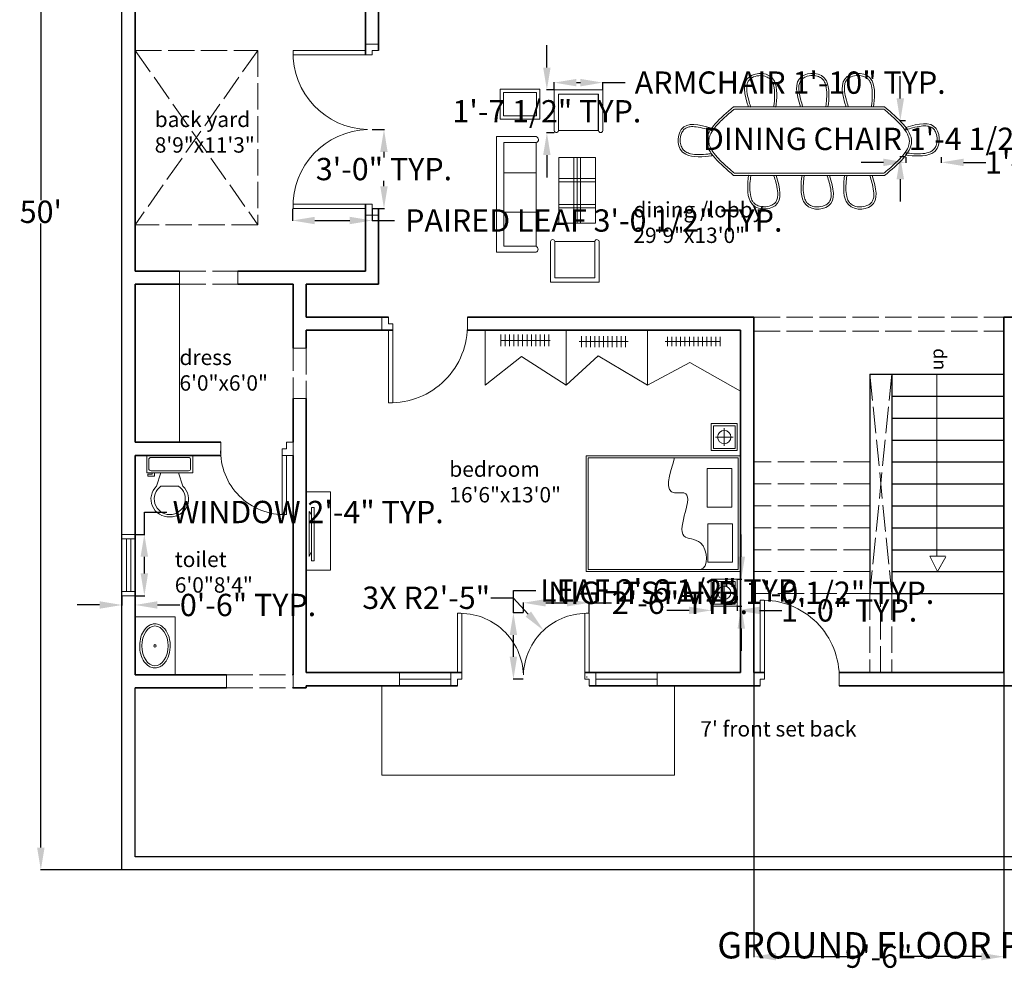
# Model space of a CAD drawing. Units: inches. Extents: x 29 to 4581, y 6 to 2196.
# Tile 1 of 3: x 3825 to 4274, y 1514 to 1948. Entities that reach past the tile are written whole.
import ezdxf

# ---------------------------------------------------------------- set-up
doc = ezdxf.new("R2010")
doc.units = ezdxf.units.IN
doc.header["$MEASUREMENT"] = 0
doc.linetypes.add('ACAD_ISO02W100', pattern=[15, 12, -3])
for name, color, linetype, lineweight in [('A-ANNO-DIMS', 2, 'Continuous', 18), ('A-ANNO-SYMB', 7, 'Continuous', 18), ('A-ANNO-TEXT', 7, 'Continuous', 25), ('A-DOOR', 3, 'Continuous', 18), ('A-EQPM', 9, 'Continuous', 18), ('A-FLOR-CASE', 8, 'Continuous', 18), ('A-FLOR-CASE-PATT', 8, 'Continuous', 13), ('A-FLOR-FIXT', 9, 'Continuous', 18), ('A-FLOR-OPEN', 8, 'ACAD_ISO02W100', 13), ('A-FLOR-STRS', 7, 'Continuous', 25), ('A-FLOR-STRS-HIDN', 8, 'ACAD_ISO02W100', 18), ('A-GLAZ', 4, 'Continuous', 18), ('A-WALL', 7, 'Continuous', 35), ('A-WALL-OVHD', 8, 'ACAD_ISO02W100', 18), ('C-PROP', 8, 'Continuous', 25), ('L-HRDS', 8, 'Continuous', 18)]:
    doc.layers.add(name, color=color, linetype=linetype, lineweight=lineweight)
doc.layers.add('A-AREA-IDEN', color=41, linetype='Continuous', lineweight=18, true_color=0xf4ee51)
doc.layers.add('A-FURN', color=31, linetype='Continuous', lineweight=18, true_color=0xfecc66)
doc.styles.get("Standard").update_dxf_attribs({"font": 'arial.ttf'})
doc.dimstyles.get("Standard").update_dxf_attribs({"dimtxt": 10.18, "dimasz": 10.18, "dimexe": 0.18, "dimexo": 0.0625, "dimgap": 0.09, "dimtad": 0, "dimtih": 1, "dimtoh": 1, "dimdec": 0, "dimzin": 0, "dimdsep": 46, "dimlunit": 3, "dimtxsty": 'Standard', "dimcen": 0.09, "dimadec": 0, "dimazin": 0, "dimtfac": 1, "dimtdec": 0, "dimtofl": 0, "dimtmove": 0, "dimatfit": 3, "dimfxl": 1, "dimtolj": 1, "dimtzin": 0, "dimarcsym": 0})

# ---------------------------------------------------------------- blocks, each defined once
blk = doc.blocks.new('*U2')
for p, q in [((9.5, -6), (9.5, -2)), ((-10, -8.5), (-8, -8.5)), ((-10, -9.5), (-10, -8.5)), ((-8, -8.5), (-8, -8)), ((-7, -8), (-7, -9.5)), ((-4, -8), (-6, -14)), ((4, -8), (6, -14)), ((-7, -9.5), (-10, -9.5)), ((4, -14), (-4, -14))]:
    blk.add_line(p, q)
blk.add_lwpolyline([(10.5, -8), (10.5, 0), (-10.5, 0), (-10.5, -8)], close=True)
for points in [[(-9.5, -2), (-9.5, -6)], [(8.5, -1), (-8.5, -1)], [(-8.5, -7), (8.5, -7)]]:
    blk.add_lwpolyline(points)
for centre, radius, start, end in [((-8.625, -1.875), 0.8839, 81.8699, 188.1301), ((8.625, -1.875), 0.8839, 351.8699, 98.1301), ((-8.625, -6.125), 0.8839, 171.869898, 278.1301), ((8.625, -6.125), 0.8839, 261.8699, 8.1301), ((-0.4772, -19.9188), 8.0953, 133.01722, 273.38), ((0.0374, -19.8731), 7.127, 124.50543, 269.7), ((-0.0373, -19.8731), 7.127, 270.3, 55.4946), ((0.4773, -19.9188), 8.0953, 266.62, 46.9828)]:
    blk.add_arc(centre, radius, start, end)
blk = doc.blocks.new('*D8')
at = {"layer": 'A-ANNO-DIMS', "color": 0, "lineweight": -2, "transparency": 16777216}
for p, q in [((3871.91, 2160.26), (3834.8, 2160.26)), ((3834.98, 2150.08), (3834.98, 1865.52)), ((3834.98, 1570.38), (3834.98, 1854.94)), ((3871.91, 1560.2), (3834.8, 1560.2))]:
    blk.add_line(p, q, dxfattribs=at)
at = {"layer": 'A-ANNO-DIMS', "color": 0, "transparency": 16777216}
for points in [[(3833.29, 2150.08), (3836.68, 2150.08), (3834.98, 2160.26)], [(3833.29, 1570.38), (3836.68, 1570.38), (3834.98, 1560.2)]]:
    blk.add_solid(points, dxfattribs=at)
at = {"layer": 'Defpoints', "color": 0, "transparency": 16777216}
for p in [(3834.98, 2160.26), (3871.98, 2160.26), (3871.98, 1560.2)]:
    blk.add_point(p, dxfattribs=at)
at = {"layer": 'A-ANNO-DIMS', "color": 0, "transparency": 16777216, "insert": (3834.98, 1860.23), "char_height": 10.18, "attachment_point": 5}
blk.add_mtext("\\A1;50'", dxfattribs=at)
blk = doc.blocks.new('CHAIR-DINING')
for p, q in [((2.81, 0.04), (1.75, 0.07)), ((13.32, 0.14), (14.31, 0))]:
    blk.add_line(p, q)
for points, knots in [([(1.75, 0.07), (0.01, 5.77), (-2.4, 15.72), (15.73, 16.36), (14.8, 3.53), (14.31, 0)], [1.303878, 1.303878, 1.303878, 1.303878, 15.362329, 26.918428, 34.974359, 34.974359, 34.974359, 34.974359]), ([(2.81, 0.04), (2.79, 0.11), (2.77, 0.18), (2.45, 1.22), (2.16, 2.19), (1.54, 4.52), (1.24, 5.86), (0.98, 8.1), (0.96, 9.04), (1.16, 10.48), (1.32, 11.03), (1.79, 11.99), (2.1, 12.41), (2.73, 12.97), (2.97, 13.14), (3.52, 13.47), (3.82, 13.62), (5.09, 14.12), (6.23, 14.34), (8.24, 14.32), (9.13, 14.17), (10.58, 13.61), (11.17, 13.26), (12, 12.49), (12.29, 12.14), (12.72, 11.45), (12.87, 11.13), (13.14, 10.42), (13.26, 10.03), (13.62, 8.47), (13.73, 7.13), (13.75, 4.38), (13.65, 2.98), (13.45, 1.15), (13.39, 0.63), (13.32, 0.14)], [1.038869, 1.038869, 1.038869, 1.038869, 1.209497, 1.209497, 3.62849, 3.62849, 7.242439, 7.242439, 10.256711, 10.256711, 12.544546, 12.544546, 14.832381, 14.832381, 15.973009, 15.973009, 17.113637, 17.113637, 20.41694, 20.41694, 23.018333, 23.018333, 25.159823, 25.159823, 26.539555, 26.539555, 27.513845, 27.513845, 28.488134, 28.488134, 31.162496, 31.162496, 33.836859, 33.836859, 34.97445, 34.97445, 34.97445, 34.97445])]:
    blk.add_open_spline(points, degree=3, knots=knots)
blk = doc.blocks.new('CHAIR-LOUNGE')
for points in [[(0, 0.82), (0, 19.42), (1.99, 19.42)], [(20.17, 19.42), (1.99, 19.42)], [(20.17, 19.42), (22.16, 19.42), (22.16, 0.82)], [(1.99, 17.47), (1.99, 0.82), (1.98, 0.82)], [(1.99, 17.47), (20.17, 17.47)], [(20.17, 0.82), (20.17, 17.47)]]:
    blk.add_lwpolyline(points)
blk.add_lwpolyline([(1.99, 17.47), (20.14, 17.47), (20.14, 0.87), (1.99, 0.87)], close=True)
for centre, radius, start, end in [((0.99, 1.01), 1.01, 190.5577, 7.8142), ((21.17, 1.03), 1.02, 191.625, 348.375)]:
    blk.add_arc(centre, radius, start, end)
blk = doc.blocks.new('DOOR-36IN')
for p, q in [((34.01, 0), (34.01, 36)), ((36.01, 3), (36.01, 36)), ((34.01, 0), (36.01, 0))]:
    blk.add_line(p, q)
blk.add_arc((35.01, 1), 35.01, 88.3634, 181.6366)
blk = doc.blocks.new('DOOR-36IN-PAIRED-LEAF')
for p, q in [((36.01, 2), (0.01, 2)), ((36.01, 2), (36.01, 0)), ((33.01, 0), (0.01, 0))]:
    blk.add_line(p, q)
blk.add_arc((35.01, 1), 35.01, 91.6366, 181.6366)
blk = doc.blocks.new('DOOR-30IN')
for p, q in [((0, 2), (30, 2)), ((0, 2), (0, 0)), ((3, 0), (30, 0))]:
    blk.add_line(p, q)
blk.add_arc((1, 1), 29.02, 358.0251, 91.9749)
blk = doc.blocks.new('DOOR-30IN-PAIRED-LEAF')
for p, q in [((28, 0), (28, 30)), ((30, 3), (30, 30)), ((28, 0), (30, 0))]:
    blk.add_line(p, q)
blk.add_arc((29, 1), 29.02, 88.0251, 178.0251)
blk = doc.blocks.new('WIN-24')
for p, q in [((6, 28), (0, 28)), ((6, 26), (0, 26)), ((2, 26), (2, 2)), ((4, 26), (4, 2)), ((6, 2), (0, 2)), ((6, 0), (0, 0))]:
    blk.add_line(p, q)
blk = doc.blocks.new('BASIN-OVAL')
blk.add_circle((10.07, 6.96), 0.572)
blk.add_ellipse((10.07, 6.96), major_axis=(9.07, 0), ratio=0.657752)
blk.add_open_spline([(20.13, 6.96), (20.13, 7.48), (20.05, 7.99), (19.74, 8.98), (19.5, 9.46), (18.6, 10.81), (17.74, 11.59), (15.67, 12.84), (14.47, 13.31), (11.89, 13.88), (10.52, 13.98), (7.83, 13.82), (6.51, 13.55), (4.11, 12.67), (3.03, 12.06), (1.49, 10.71), (0.93, 10.02), (0.24, 8.64), (0.05, 7.96), (-0.03, 6.59), (0.07, 5.9), (0.54, 4.6), (0.91, 3.98), (1.85, 2.86), (2.43, 2.36), (4.23, 1.16), (5.63, 0.61), (8.62, -0.01), (10.22, -0.08), (13.3, 0.28), (14.78, 0.7), (17.33, 1.99), (18.39, 2.86), (19.54, 4.5), (19.85, 5.16), (20.09, 6.22), (20.13, 6.59), (20.13, 6.96)], degree=3, knots=[0, 0, 0, 0, 0.206246, 0.206246, 0.412492, 0.412492, 0.829146, 0.829146, 1.245799, 1.245799, 1.662453, 1.662453, 2.079106, 2.079106, 2.495759, 2.495759, 2.824502, 2.824502, 3.099346, 3.099346, 3.37419, 3.37419, 3.649034, 3.649034, 3.923877, 3.923877, 4.405635, 4.405635, 4.887392, 4.887392, 5.369149, 5.369149, 5.850906, 5.850906, 6.134068, 6.134068, 6.283185, 6.283185, 6.283185, 6.283185])
blk = doc.blocks.new('NIGHTSTAND-NARROW')
for p, q in [((5.9, 10.31), (5.9, 2.16)), ((1.96, 6.19), (10.01, 6.19))]:
    blk.add_line(p, q)
for points in [[(0, 12.38), (11.8, 12.38), (11.8, 0), (0, 0)], [(1, 11.38), (10.8, 11.38), (10.8, 1), (1, 1)]]:
    blk.add_lwpolyline(points, close=True)
blk.add_circle((5.9, 6.19), 3.03)
blk = doc.blocks.new('*D22')
at = {"layer": 'A-ANNO-DIMS', "color": 0, "lineweight": -2, "transparency": 16777216}
for p, q in [((4226.82, 1911.89), (4226.82, 1922.07)), ((4229.23, 1901.71), (4226.64, 1901.71)), ((4229.23, 1885.22), (4226.64, 1885.22)), ((4226.82, 1875.04), (4226.82, 1864.86))]:
    blk.add_line(p, q, dxfattribs=at)
at = {"layer": 'A-ANNO-DIMS', "color": 0, "transparency": 16777216}
for points in [[(4225.13, 1911.89), (4228.52, 1911.89), (4226.82, 1901.71)], [(4225.13, 1875.04), (4228.52, 1875.04), (4226.82, 1885.22)]]:
    blk.add_solid(points, dxfattribs=at)
at = {"layer": 'Defpoints', "color": 0, "transparency": 16777216}
for p in [(4229.3, 1901.71), (4226.82, 1885.22), (4229.3, 1885.22)]:
    blk.add_point(p, dxfattribs=at)
at = {"layer": 'A-ANNO-DIMS', "color": 0, "transparency": 16777216, "insert": (4226.82, 1893.47), "char_height": 10.18, "attachment_point": 5}
blk.add_mtext('\\A1;DINING CHAIR 1\'-4 1/2" TYP.', dxfattribs=at)
blk = doc.blocks.new('*D23')
at = {"layer": 'A-ANNO-DIMS', "color": 0, "lineweight": -2, "transparency": 16777216}
for p, q in [((4219.12, 1882.74), (4208.94, 1882.74)), ((4229.3, 1885.16), (4229.3, 1882.56)), ((4245.51, 1885.16), (4245.51, 1882.56)), ((4255.69, 1882.74), (4265.87, 1882.74))]:
    blk.add_line(p, q, dxfattribs=at)
at = {"layer": 'A-ANNO-DIMS', "color": 0, "transparency": 16777216}
for points in [[(4219.12, 1884.44), (4219.12, 1881.05), (4229.3, 1882.74)], [(4255.69, 1884.44), (4255.69, 1881.05), (4245.51, 1882.74)]]:
    blk.add_solid(points, dxfattribs=at)
at = {"layer": 'Defpoints', "color": 0, "transparency": 16777216}
for p in [(4229.3, 1885.22), (4245.51, 1885.22), (4245.51, 1882.74)]:
    blk.add_point(p, dxfattribs=at)
at = {"layer": 'A-ANNO-DIMS', "color": 0, "transparency": 16777216, "insert": (4296.5, 1882.74), "char_height": 10.18, "attachment_point": 5}
blk.add_mtext('\\A1;1\'-4" TYP.', dxfattribs=at)
blk = doc.blocks.new('*D30')
at = {"layer": 'A-ANNO-DIMS', "color": 0, "lineweight": -2, "transparency": 16777216}
for p, q in [((3949.71, 1861.63), (3949.71, 1856.08)), ((3985.98, 1861.63), (3985.98, 1856.08)), ((3959.89, 1856.26), (3975.8, 1856.26)), ((3985.98, 1856.26), (3996.16, 1856.26))]:
    blk.add_line(p, q, dxfattribs=at)
at = {"layer": 'A-ANNO-DIMS', "color": 0, "transparency": 16777216}
for points in [[(3959.89, 1857.95), (3959.89, 1854.56), (3949.71, 1856.26)], [(3975.8, 1857.95), (3975.8, 1854.56), (3985.98, 1856.26)]]:
    blk.add_solid(points, dxfattribs=at)
at = {"layer": 'Defpoints', "color": 0, "transparency": 16777216}
for p in [(3949.71, 1861.7), (3985.98, 1861.7), (3985.98, 1856.26)]:
    blk.add_point(p, dxfattribs=at)
at = {"layer": 'A-ANNO-DIMS', "color": 0, "transparency": 16777216, "insert": (4087.09, 1856.26), "char_height": 10.18, "attachment_point": 5}
blk.add_mtext('\\A1;PAIRED LEAF 3\'-0 1/2" TYP.', dxfattribs=at)
blk = doc.blocks.new('*D31')
at = {"layer": 'A-ANNO-DIMS', "color": 0, "lineweight": -2, "transparency": 16777216}
for p, q in [((3986.04, 1897.7), (3991.6, 1897.7)), ((3991.42, 1887.52), (3991.42, 1884.99)), ((3991.42, 1871.88), (3991.42, 1874.41)), ((3986.04, 1861.7), (3991.6, 1861.7))]:
    blk.add_line(p, q, dxfattribs=at)
at = {"layer": 'A-ANNO-DIMS', "color": 0, "transparency": 16777216}
for points in [[(3989.72, 1887.52), (3993.11, 1887.52), (3991.42, 1897.7)], [(3989.72, 1871.88), (3993.11, 1871.88), (3991.42, 1861.7)]]:
    blk.add_solid(points, dxfattribs=at)
at = {"layer": 'Defpoints', "color": 0, "transparency": 16777216}
for p in [(3985.98, 1897.7), (3991.42, 1897.7), (3985.98, 1861.7)]:
    blk.add_point(p, dxfattribs=at)
at = {"layer": 'A-ANNO-DIMS', "color": 0, "transparency": 16777216, "insert": (3991.42, 1879.7), "char_height": 10.18, "attachment_point": 5}
blk.add_mtext('\\A1;3\'-0" TYP.', dxfattribs=at)
blk = doc.blocks.new('*D32')
at = {"layer": 'A-ANNO-DIMS', "color": 0, "lineweight": -2, "transparency": 16777216}
for p, q in [((3882.18, 1713.2), (3882.18, 1723.38)), ((3882.18, 1723.38), (3892.36, 1723.38)), ((3878.04, 1713.2), (3882.36, 1713.2)), ((3882.18, 1695.38), (3882.18, 1703.02)), ((3878.04, 1685.2), (3882.36, 1685.2))]:
    blk.add_line(p, q, dxfattribs=at)
at = {"layer": 'A-ANNO-DIMS', "color": 0, "transparency": 16777216}
for points in [[(3880.48, 1703.02), (3883.87, 1703.02), (3882.18, 1713.2)], [(3880.48, 1695.38), (3883.87, 1695.38), (3882.18, 1685.2)]]:
    blk.add_solid(points, dxfattribs=at)
at = {"layer": 'Defpoints', "color": 0, "transparency": 16777216}
for p in [(3877.98, 1713.2), (3882.18, 1713.2), (3877.98, 1685.2)]:
    blk.add_point(p, dxfattribs=at)
at = {"layer": 'A-ANNO-DIMS', "color": 0, "transparency": 16777216, "insert": (3956.86, 1723.38), "char_height": 10.18, "attachment_point": 5}
blk.add_mtext('\\A1;WINDOW 2\'-4" TYP.', dxfattribs=at)
blk = doc.blocks.new('*D33')
at = {"layer": 'A-ANNO-DIMS', "color": 0, "lineweight": -2, "transparency": 16777216}
for p, q in [((3871.98, 1685.13), (3871.98, 1680.82)), ((3877.98, 1685.13), (3877.98, 1680.82)), ((3861.8, 1681), (3851.62, 1681)), ((3888.16, 1681), (3898.34, 1681))]:
    blk.add_line(p, q, dxfattribs=at)
at = {"layer": 'A-ANNO-DIMS', "color": 0, "transparency": 16777216}
for points in [[(3861.8, 1682.69), (3861.8, 1679.3), (3871.98, 1681)], [(3888.16, 1682.69), (3888.16, 1679.3), (3877.98, 1681)]]:
    blk.add_solid(points, dxfattribs=at)
at = {"layer": 'Defpoints', "color": 0, "transparency": 16777216}
for p in [(3871.98, 1685.2), (3877.98, 1685.2), (3877.98, 1681)]:
    blk.add_point(p, dxfattribs=at)
at = {"layer": 'A-ANNO-DIMS', "color": 0, "transparency": 16777216, "insert": (3929.45, 1681), "char_height": 10.18, "attachment_point": 5}
blk.add_mtext('\\A1;0\'-6" TYP.', dxfattribs=at)
blk = doc.blocks.new('*D36')
at = {"layer": 'A-ANNO-DIMS', "color": 0, "lineweight": -2, "transparency": 16777216}
for p, q in [((4069.01, 1915.84), (4069.01, 1919.29)), ((4079.19, 1919.11), (4081, 1919.11)), ((4091.18, 1915.84), (4091.18, 1919.29)), ((4091.18, 1919.11), (4101.36, 1919.11))]:
    blk.add_line(p, q, dxfattribs=at)
at = {"layer": 'A-ANNO-DIMS', "color": 0, "transparency": 16777216}
for points in [[(4079.19, 1920.8), (4079.19, 1917.41), (4069.01, 1919.11)], [(4081, 1920.8), (4081, 1917.41), (4091.18, 1919.11)]]:
    blk.add_solid(points, dxfattribs=at)
at = {"layer": 'Defpoints', "color": 0, "transparency": 16777216}
for p in [(4091.18, 1919.11), (4069.01, 1915.78), (4091.18, 1915.78)]:
    blk.add_point(p, dxfattribs=at)
at = {"layer": 'A-ANNO-DIMS', "color": 0, "transparency": 16777216, "insert": (4176.62, 1919.11), "char_height": 10.18, "attachment_point": 5}
blk.add_mtext('\\A1;ARMCHAIR 1\'-10" TYP.', dxfattribs=at)
blk = doc.blocks.new('*D37')
at = {"layer": 'A-ANNO-DIMS', "color": 0, "lineweight": -2, "transparency": 16777216}
for p, q in [((4065.69, 1925.96), (4065.69, 1936.14)), ((4068.95, 1915.78), (4065.51, 1915.78)), ((4068.95, 1896.29), (4065.51, 1896.29)), ((4065.69, 1886.11), (4065.69, 1875.93))]:
    blk.add_line(p, q, dxfattribs=at)
at = {"layer": 'A-ANNO-DIMS', "color": 0, "transparency": 16777216}
for points in [[(4063.99, 1925.96), (4067.38, 1925.96), (4065.69, 1915.78)], [(4063.99, 1886.11), (4067.38, 1886.11), (4065.69, 1896.29)]]:
    blk.add_solid(points, dxfattribs=at)
at = {"layer": 'Defpoints', "color": 0, "transparency": 16777216}
for p in [(4065.69, 1915.78), (4069.01, 1915.78), (4069.01, 1896.29)]:
    blk.add_point(p, dxfattribs=at)
at = {"layer": 'A-ANNO-DIMS', "color": 0, "transparency": 16777216, "insert": (4065.69, 1906.04), "char_height": 10.18, "attachment_point": 5}
blk.add_mtext('\\A1;1\'-7 1/2" TYP.', dxfattribs=at)
blk = doc.blocks.new('*D38')
at = {"layer": 'A-ANNO-DIMS', "color": 0, "lineweight": -2, "transparency": 16777216}
for p, q in [((4050.44, 1677.46), (4050.44, 1687.64)), ((4050.44, 1687.64), (4060.62, 1687.64)), ((4054.91, 1677.46), (4050.26, 1677.46)), ((4050.44, 1657.38), (4050.44, 1667.28)), ((4054.91, 1647.2), (4050.26, 1647.2))]:
    blk.add_line(p, q, dxfattribs=at)
at = {"layer": 'A-ANNO-DIMS', "color": 0, "transparency": 16777216}
for points in [[(4048.74, 1667.28), (4052.13, 1667.28), (4050.44, 1677.46)], [(4048.74, 1657.38), (4052.13, 1657.38), (4050.44, 1647.2)]]:
    blk.add_solid(points, dxfattribs=at)
at = {"layer": 'Defpoints', "color": 0, "transparency": 16777216}
for p in [(4050.44, 1677.46), (4054.98, 1677.46), (4054.98, 1647.2)]:
    blk.add_point(p, dxfattribs=at)
at = {"layer": 'A-ANNO-DIMS', "color": 0, "transparency": 16777216, "insert": (4123.13, 1687.64), "char_height": 10.18, "attachment_point": 5}
blk.add_mtext('\\A1;LEAF 2\'-6 1/2" TYP.', dxfattribs=at)
blk = doc.blocks.new('*D39')
at = {"layer": 'A-ANNO-DIMS', "color": 0, "lineweight": -2, "transparency": 16777216}
for p, q in [((4054.98, 1677.52), (4054.98, 1682.18)), ((4065.16, 1682), (4074.8, 1682)), ((4084.98, 1677.52), (4084.98, 1682.18)), ((4084.98, 1682), (4095.16, 1682))]:
    blk.add_line(p, q, dxfattribs=at)
at = {"layer": 'A-ANNO-DIMS', "color": 0, "transparency": 16777216}
for points in [[(4065.16, 1683.7), (4065.16, 1680.31), (4054.98, 1682)], [(4074.8, 1683.7), (4074.8, 1680.31), (4084.98, 1682)]]:
    blk.add_solid(points, dxfattribs=at)
at = {"layer": 'Defpoints', "color": 0, "transparency": 16777216}
for p in [(4084.98, 1682), (4054.98, 1677.46), (4084.98, 1677.46)]:
    blk.add_point(p, dxfattribs=at)
at = {"layer": 'A-ANNO-DIMS', "color": 0, "transparency": 16777216, "insert": (4126.36, 1682), "char_height": 10.18, "attachment_point": 5}
blk.add_mtext('\\A1;2\'-6" TYP.', dxfattribs=at)
blk = doc.blocks.new('*D42')
at = {"layer": 'A-ANNO-DIMS', "color": 0, "lineweight": -2, "transparency": 16777216}
for p, q in [((4154.32, 1702.95), (4154.32, 1713.13)), ((4152.53, 1692.77), (4154.5, 1692.77)), ((4152.53, 1680.39), (4154.5, 1680.39)), ((4154.32, 1670.21), (4154.32, 1660.03))]:
    blk.add_line(p, q, dxfattribs=at)
at = {"layer": 'A-ANNO-DIMS', "color": 0, "transparency": 16777216}
for points in [[(4152.63, 1702.95), (4156.02, 1702.95), (4154.32, 1692.77)], [(4152.63, 1670.21), (4156.02, 1670.21), (4154.32, 1680.39)]]:
    blk.add_solid(points, dxfattribs=at)
at = {"layer": 'Defpoints', "color": 0, "transparency": 16777216}
for p in [(4152.47, 1692.77), (4154.32, 1692.77), (4152.47, 1680.39)]:
    blk.add_point(p, dxfattribs=at)
at = {"layer": 'A-ANNO-DIMS', "color": 0, "transparency": 16777216, "insert": (4154.32, 1686.58), "char_height": 10.18, "attachment_point": 5}
blk.add_mtext('\\A1;NIGHTSTAND 1\'-0 1/2" TYP.', dxfattribs=at)
blk = doc.blocks.new('*D43')
at = {"layer": 'A-ANNO-DIMS', "color": 0, "lineweight": -2, "transparency": 16777216}
for p, q in [((4140.67, 1680.33), (4140.67, 1678.35)), ((4152.47, 1680.33), (4152.47, 1678.35)), ((4130.49, 1678.53), (4120.31, 1678.53)), ((4162.65, 1678.53), (4172.83, 1678.53))]:
    blk.add_line(p, q, dxfattribs=at)
at = {"layer": 'A-ANNO-DIMS', "color": 0, "transparency": 16777216}
for points in [[(4130.49, 1680.23), (4130.49, 1676.83), (4140.67, 1678.53)], [(4162.65, 1680.23), (4162.65, 1676.83), (4152.47, 1678.53)]]:
    blk.add_solid(points, dxfattribs=at)
at = {"layer": 'Defpoints', "color": 0, "transparency": 16777216}
for p in [(4140.67, 1680.39), (4152.47, 1680.39), (4152.47, 1678.53)]:
    blk.add_point(p, dxfattribs=at)
at = {"layer": 'A-ANNO-DIMS', "color": 0, "transparency": 16777216, "insert": (4203.46, 1678.53), "char_height": 10.18, "attachment_point": 5}
blk.add_mtext('\\A1;1\'-0" TYP.', dxfattribs=at)
blk = doc.blocks.new('*D47')
at = {"layer": 'A-ANNO-DIMS', "color": 0, "lineweight": -2, "transparency": 16777216}
for p, q in [((4159.98, 1650.13), (4159.98, 1520.52)), ((4273.98, 1650.13), (4273.98, 1520.52)), ((4170.16, 1520.7), (4203.36, 1520.7)), ((4263.8, 1520.7), (4230.6, 1520.7))]:
    blk.add_line(p, q, dxfattribs=at)
at = {"layer": 'A-ANNO-DIMS', "color": 0, "transparency": 16777216}
for points in [[(4170.16, 1522.39), (4170.16, 1519), (4159.98, 1520.7)], [(4263.8, 1522.39), (4263.8, 1519), (4273.98, 1520.7)]]:
    blk.add_solid(points, dxfattribs=at)
at = {"layer": 'Defpoints', "color": 0, "transparency": 16777216}
for p in [(4159.98, 1650.2), (4273.98, 1650.2), (4273.98, 1520.7)]:
    blk.add_point(p, dxfattribs=at)
at = {"layer": 'A-ANNO-DIMS', "color": 0, "transparency": 16777216, "insert": (4216.98, 1520.7), "char_height": 10.18, "attachment_point": 5}
blk.add_mtext('\\A1;9\'-6"', dxfattribs=at)
blk = doc.blocks.new('*D49')
at = {"layer": 'A-ANNO-DIMS', "color": 0, "lineweight": -2, "transparency": 16777216}
for p, q in [((4040.11, 1684.29), (4050.29, 1684.29)), ((4050.29, 1684.29), (4057.23, 1676.85)), ((4083.89, 1648.2), (4084.07, 1648.2)), ((4083.98, 1648.11), (4083.98, 1648.29))]:
    blk.add_line(p, q, dxfattribs=at)
at = {"layer": 'A-ANNO-DIMS', "color": 0, "transparency": 16777216}
blk.add_solid([(4058.47, 1678.01), (4055.99, 1675.69), (4064.18, 1669.41)], dxfattribs=at)
at = {"layer": 'Defpoints', "color": 0, "transparency": 16777216}
for p in [(4064.18, 1669.41), (4083.98, 1648.2)]:
    blk.add_point(p, dxfattribs=at)
at = {"layer": 'A-ANNO-DIMS', "color": 0, "transparency": 16777216, "insert": (4010.68, 1684.29), "char_height": 10.18, "attachment_point": 5}
blk.add_mtext('\\A1;3X R2\'-5"', dxfattribs=at)

msp = doc.modelspace()

# ---------------------------------------------------------------- hatches: boundary and pattern name
at = {"layer": 'A-FLOR-CASE-PATT'}
h = msp.add_hatch(dxfattribs=at)
h.set_pattern_fill('ANSI31', color=256, scale=16.00257, angle=45, style=0)
h.paths.add_polyline_path([(4043.65, 1798.98), (4067.65, 1798.98), (4067.65, 1804.28), (4043.65, 1804.28)])
h = msp.add_hatch(dxfattribs=at)
h.set_pattern_fill('ANSI31', color=256, scale=15.99816, angle=45, style=0)
h.paths.add_polyline_path([(4080.53, 1798.52), (4102.53, 1798.52), (4102.53, 1803.55), (4080.53, 1803.55)])
h = msp.add_hatch(dxfattribs=at)
h.set_pattern_fill('ANSI31', color=256, scale=16.00254, angle=45, style=0)
h.paths.add_polyline_path([(4119.65, 1798.9), (4145.65, 1798.9), (4145.65, 1803.26), (4119.65, 1803.26)])

# ---------------------------------------------------------------- linework, layer by layer
at = {"layer": 'A-ANNO-SYMB'}
for p, q in [((4243.46, 1786.2), (4243.46, 1703.22)), ((4247.45, 1703.22), (4240.33, 1703.22)), ((4240.33, 1703.22), (4243.75, 1696.2)), ((4243.46, 1703.22), (4247.45, 1703.22)), ((4243.75, 1696.2), (4247.63, 1702.91))]:
    msp.add_line(p, q, dxfattribs=at)
at = {"layer": 'A-DOOR'}
for p, q in [((3988.98, 1936.7), (3982.98, 1936.7)), ((3988.98, 1933.7), (3985.98, 1933.7)), ((3982.98, 1897.65), (3982.98, 1897.74)), ((3983.98, 1897.7), (3982.98, 1897.7)), ((3988.98, 1858.7), (3982.98, 1858.7)), ((3988.98, 1861.7), (3985.98, 1861.7)), ((3990.45, 1812.2), (3990.45, 1806.2)), ((3993.45, 1812.2), (3993.45, 1809.2)), ((4029.45, 1812.2), (4029.45, 1806.2)), ((3916.98, 1755.2), (3916.98, 1749.2)), ((3946.98, 1755.2), (3946.98, 1752.2)), ((3946.98, 1755.2), (3949.98, 1755.2)), ((3949.98, 1755.2), (3949.98, 1749.2)), ((3944.98, 1749.2), (3949.98, 1749.2)), ((4021.98, 1650.2), (4021.98, 1644.2)), ((4054.92, 1650.2), (4055.03, 1650.2)), ((4054.98, 1650.2), (4054.98, 1649.2)), ((4087.98, 1650.2), (4087.98, 1644.2)), ((4159.98, 1650.2), (4159.98, 1644.2)), ((4198.98, 1650.2), (4198.98, 1644.2)), ((4024.98, 1647.2), (4024.98, 1644.2)), ((4084.98, 1647.2), (4084.98, 1644.2)), ((4162.98, 1647.2), (4162.98, 1644.2))]:
    msp.add_line(p, q, dxfattribs=at)
at = {"layer": 'A-EQPM'}
for p, q in [((3958.45, 1722.26), (3957.35, 1723.66)), ((3957.35, 1723.66), (3957.35, 1703.05)), ((3957.35, 1703.05), (3958.45, 1705.42))]:
    msp.add_line(p, q, dxfattribs=at)
for points in [[(3955.98, 1732.54), (3966.99, 1732.54), (3966.99, 1696.8), (3955.98, 1696.8)], [(3958.45, 1725.42), (3959.67, 1725.42), (3959.67, 1701.19), (3958.45, 1701.19)]]:
    msp.add_lwpolyline(points, close=True, dxfattribs=at)
at = {"layer": 'A-FLOR-CASE'}
for p, q in [((3898.19, 1827.2), (3898.19, 1755.2)), ((4037.56, 1806.2), (4037.56, 1781.27)), ((4074.47, 1806.2), (4074.47, 1781.27)), ((4111.62, 1806.2), (4111.62, 1781.27)), ((4044.69, 1801.59), (4067.16, 1801.59)), ((4080.34, 1801.1), (4102.81, 1801.1)), ((4119.58, 1801.1), (4144.65, 1801.1)), ((4037.56, 1781.27), (4054.12, 1794.2)), ((4054.12, 1794.2), (4074.47, 1781.27)), ((4074.47, 1781.27), (4089.07, 1794.62)), ((4089.07, 1794.62), (4111.62, 1781.27)), ((4111.62, 1781.27), (4130.86, 1791.58)), ((4130.86, 1791.58), (4153.98, 1778.52))]:
    msp.add_line(p, q, dxfattribs=at)
at = {"layer": 'A-FLOR-FIXT'}
for p, q in [((3877.98, 1675.67), (3896.27, 1675.67)), ((3896.27, 1675.67), (3896.27, 1649.2))]:
    msp.add_line(p, q, dxfattribs=at)
at = {"layer": 'A-FLOR-OPEN'}
for p, q in [((3877.98, 1933.81), (3933.88, 1933.81)), ((3877.98, 1933.81), (3933.88, 1854.3)), ((3933.88, 1933.81), (3877.98, 1854.3)), ((3933.88, 1933.81), (3933.88, 1854.3)), ((3933.88, 1854.3), (3877.98, 1854.3))]:
    msp.add_line(p, q, dxfattribs=at)
at = {"layer": 'A-FLOR-STRS'}
for p, q in [((4212.95, 1786.2), (4273.98, 1786.2)), ((4212.95, 1786.2), (4212.95, 1686.2)), ((4222.95, 1786.2), (4222.95, 1686.2)), ((4222.95, 1776.2), (4273.98, 1776.2)), ((4222.95, 1766.2), (4273.98, 1766.2)), ((4222.95, 1756.2), (4273.98, 1756.2)), ((4222.95, 1746.2), (4273.98, 1746.2)), ((4222.95, 1736.2), (4273.98, 1736.2)), ((4222.95, 1726.2), (4273.98, 1726.2)), ((4222.95, 1716.2), (4273.98, 1716.2)), ((4222.95, 1706.2), (4273.98, 1706.2)), ((4222.95, 1696.2), (4273.98, 1696.2))]:
    msp.add_line(p, q, dxfattribs=at)
msp.add_lwpolyline([(4212.95, 1686.2), (4273.98, 1686.2)], dxfattribs=at)
at = {"layer": 'A-FLOR-STRS-HIDN'}
for p, q in [((4212.95, 1786.2), (4222.95, 1686.2)), ((4222.95, 1786.2), (4212.95, 1686.2)), ((4212.95, 1746.2), (4159.98, 1746.2)), ((4212.95, 1736.2), (4159.98, 1736.2)), ((4212.95, 1726.2), (4159.98, 1726.2)), ((4212.95, 1716.2), (4159.98, 1716.2)), ((4212.95, 1706.2), (4159.98, 1706.2)), ((4212.95, 1696.2), (4159.98, 1696.2)), ((4212.95, 1686.2), (4159.98, 1686.2)), ((4212.95, 1686.2), (4212.95, 1650.2)), ((4217.79, 1650.2), (4217.79, 1686.2)), ((4222.95, 1686.2), (4222.95, 1650.2))]:
    msp.add_line(p, q, dxfattribs=at)
at = {"layer": 'A-FURN'}
for p, q in [((4150.84, 1908.06), (4219.67, 1908.06)), ((4151.21, 1907.06), (4219.3, 1907.06)), ((4077.99, 1884.92), (4077.99, 1855.04)), ((4079.52, 1884.92), (4079.52, 1855.04)), ((4081.04, 1884.92), (4081.04, 1855.04)), ((4046.01, 1878.02), (4060.88, 1878.02)), ((4150.84, 1876.77), (4219.58, 1876.77)), ((4151.21, 1877.77), (4219.3, 1877.77)), ((4071.16, 1875.4), (4087.87, 1875.4)), ((4071.16, 1873.88), (4087.87, 1873.88)), ((4071.16, 1863.48), (4087.87, 1863.48)), ((4046.01, 1860.08), (4060.88, 1860.08)), ((4071.16, 1861.96), (4087.87, 1861.96))]:
    msp.add_line(p, q, dxfattribs=at)
for points in [[(4044.37, 1916.1), (4062.53, 1916.1), (4062.53, 1902.39), (4044.37, 1902.39)], [(4045.9, 1914.58), (4061.01, 1914.58), (4061.01, 1903.91), (4045.9, 1903.91)], [(4060.88, 1891.83), (4046.01, 1891.83), (4046.01, 1844.49), (4060.88, 1844.49)], [(4071.16, 1884.92), (4087.87, 1884.92), (4087.87, 1855.04), (4071.16, 1855.04)], [(4153.98, 1749.03), (4083.55, 1749.03), (4083.55, 1696.2), (4153.98, 1696.2)], [(4152.98, 1748.03), (4084.55, 1748.03), (4084.55, 1697.2), (4152.98, 1697.2)], [(4150.06, 1743.16), (4138.76, 1743.16), (4138.76, 1725.66), (4150.06, 1725.66)], [(4150.34, 1718.02), (4139.05, 1718.02), (4139.05, 1700.51), (4150.34, 1700.51)]]:
    msp.add_lwpolyline(points, close=True, dxfattribs=at)
for points in [[(4060.8, 1894.48), (4042.71, 1894.48), (4042.71, 1891.83)], [(4042.71, 1891.83), (4042.71, 1844.51)], [(4046.01, 1844.51), (4046.01, 1891.83)], [(4046.01, 1891.83), (4060.8, 1891.83)], [(4042.71, 1844.46), (4042.71, 1841.81), (4060.8, 1841.81)]]:
    msp.add_lwpolyline(points, dxfattribs=at)
for centre, radius, start, end in [((4060.51, 1893.14), 1.37, 285.567, 77.603), ((4060.26, 1843.13), 1.43, 292.0951, 67.9049)]:
    msp.add_arc(centre, radius, start, end, dxfattribs=at)
for points, knots in [([(4150.84, 1908.06), (4144.72, 1902.92), (4132.4, 1892.56), (4144.66, 1882.06), (4150.84, 1876.77)], [0, 0, 0, 0, 19.754281, 39.795573, 39.795573, 39.795573, 39.795573]), ([(4219.67, 1876.77), (4225.79, 1881.91), (4238.11, 1892.27), (4225.85, 1902.77), (4219.67, 1908.06)], [0, 0, 0, 0, 19.754281, 39.795573, 39.795573, 39.795573, 39.795573]), ([(4151.21, 1907.06), (4150.83, 1906.75), (4150.46, 1906.44), (4149.17, 1905.35), (4148.26, 1904.57), (4145.65, 1902.25), (4144.04, 1900.71), (4141.79, 1898.07), (4141, 1896.96), (4140.04, 1895.07), (4139.76, 1894.28), (4139.54, 1892.94), (4139.52, 1892.38), (4139.66, 1891.25), (4139.81, 1890.67), (4140.46, 1888.96), (4141.16, 1887.79), (4142.99, 1885.42), (4144.12, 1884.21), (4146.63, 1881.77), (4148.01, 1880.53), (4150.02, 1878.79), (4150.62, 1878.28), (4151.21, 1877.77)], [0.300401, 0.300401, 0.300401, 0.300401, 1.50128, 1.50128, 4.50384, 4.50384, 10.50896, 10.50896, 14.992454, 14.992454, 18.387915, 18.387915, 20.903363, 20.903363, 23.41881, 23.41881, 28.133149, 28.133149, 32.847488, 32.847488, 37.561826, 37.561826, 39.491832, 39.491832, 39.491832, 39.491832]), ([(4219.3, 1877.77), (4219.68, 1878.08), (4220.05, 1878.4), (4221.34, 1879.49), (4222.24, 1880.26), (4224.86, 1882.59), (4226.47, 1884.12), (4228.72, 1886.76), (4229.51, 1887.87), (4230.47, 1889.76), (4230.75, 1890.56), (4230.97, 1891.9), (4230.99, 1892.45), (4230.85, 1893.59), (4230.7, 1894.17), (4230.05, 1895.88), (4229.35, 1897.04), (4227.52, 1899.42), (4226.39, 1900.63), (4223.88, 1903.07), (4222.5, 1904.3), (4220.49, 1906.05), (4219.89, 1906.55), (4219.3, 1907.06)], [0.300401, 0.300401, 0.300401, 0.300401, 1.50128, 1.50128, 4.50384, 4.50384, 10.50896, 10.50896, 14.992454, 14.992454, 18.387915, 18.387915, 20.903363, 20.903363, 23.41881, 23.41881, 28.133149, 28.133149, 32.847488, 32.847488, 37.561826, 37.561826, 39.491832, 39.491832, 39.491832, 39.491832]), ([(4123.95, 1748.03), (4121.52, 1740.3), (4118.45, 1730.53), (4135.37, 1734.1), (4120.76, 1709.88), (4138.95, 1712.01), (4139.58, 1696.89), (4135.01, 1697.18), (4134.6, 1697.2)], [0, 0, 0, 0, 15.945731, 20.155624, 39.777324, 48.05002, 60.112236, 61.298077, 61.298077, 61.298077, 61.298077])]:
    msp.add_open_spline(points, degree=3, knots=knots, dxfattribs=at)
at = {"layer": 'A-GLAZ'}
for p, q in [((3998.54, 1650.2), (3998.54, 1644.2)), ((4115.9, 1650.2), (4115.9, 1644.2)), ((3998.54, 1647.2), (4021.98, 1647.2)), ((4087.98, 1647.2), (4115.9, 1647.2))]:
    msp.add_line(p, q, dxfattribs=at)
at = {"layer": 'A-WALL'}
for p, q in [((3877.98, 1833.2), (3877.98, 1968.2)), ((3982.98, 1931.7), (3982.98, 1968.2)), ((3988.98, 1933.7), (3988.98, 1968.2)), ((3982.98, 1833.2), (3982.98, 1863.7)), ((3988.98, 1827.2), (3988.98, 1861.7)), ((3877.98, 1833.2), (3898.19, 1833.2)), ((3924.79, 1833.2), (3982.98, 1833.2)), ((3877.98, 1827.2), (3898.19, 1827.2)), ((3877.98, 1755.2), (3877.98, 1827.2)), ((3924.79, 1827.2), (3949.98, 1827.2)), ((3949.98, 1798.12), (3949.98, 1827.2)), ((3955.98, 1827.2), (3988.98, 1827.2)), ((3955.98, 1812.2), (3955.98, 1827.2)), ((3955.98, 1812.2), (3993.45, 1812.2)), ((4029.45, 1812.2), (4159.98, 1812.2)), ((4159.98, 1650.2), (4159.98, 1812.2)), ((4273.98, 1812.2), (4273.98, 1650.2)), ((4273.98, 1812.2), (4282.98, 1812.2)), ((3955.98, 1806.2), (3995.45, 1806.2)), ((3955.98, 1798.12), (3955.98, 1806.2)), ((4029.41, 1806.2), (4153.98, 1806.2)), ((4153.98, 1650.2), (4153.98, 1806.2)), ((3949.98, 1755.2), (3949.98, 1775.09)), ((3955.98, 1749.2), (3955.98, 1775.09)), ((3877.98, 1755.2), (3916.98, 1755.2)), ((3877.98, 1749.2), (3917.03, 1749.2)), ((3877.98, 1649.2), (3877.98, 1749.2)), ((3949.98, 1649.2), (3949.98, 1749.2)), ((3955.98, 1650.2), (3955.98, 1749.2)), ((3877.98, 1649.2), (3919.6, 1649.2)), ((3955.98, 1650.2), (4026.98, 1650.2)), ((4082.98, 1650.2), (4153.98, 1650.2)), ((4159.98, 1650.2), (4164.98, 1650.2)), ((4198.93, 1650.2), (4273.98, 1650.2)), ((3877.98, 1643.2), (3919.6, 1643.2)), ((3949.98, 1643.2), (3955.98, 1643.2)), ((3955.98, 1643.2), (3955.98, 1644.2)), ((3955.98, 1644.2), (4024.98, 1644.2)), ((4084.98, 1644.2), (4162.98, 1644.2)), ((4198.98, 1644.2), (4429.98, 1644.2))]:
    msp.add_line(p, q, dxfattribs=at)
at = {"layer": 'A-WALL-OVHD'}
for p, q in [((3898.19, 1833.2), (3898.19, 1827.2)), ((3898.19, 1833.2), (3924.79, 1833.2)), ((3924.79, 1833.2), (3924.79, 1827.2)), ((3898.19, 1827.2), (3924.79, 1827.2)), ((4159.98, 1812.2), (4273.98, 1812.2)), ((4159.98, 1805.85), (4273.98, 1805.85)), ((3949.98, 1799.67), (3949.98, 1775.09)), ((3955.98, 1798.12), (3949.98, 1798.12)), ((3955.98, 1798.12), (3955.98, 1775.09)), ((3949.98, 1775.09), (3955.98, 1775.09)), ((3919.6, 1649.2), (3919.6, 1643.2)), ((3919.6, 1649.2), (3949.98, 1649.2)), ((3949.98, 1649.2), (3949.98, 1643.2)), ((3919.6, 1643.2), (3949.98, 1643.2))]:
    msp.add_line(p, q, dxfattribs=at)
at = {"layer": 'C-PROP'}
for p, q in [((3871.98, 1560.2), (3871.98, 2160.2)), ((3877.98, 1566.2), (3877.98, 1643.2)), ((4437.42, 1566.2), (3877.98, 1566.2)), ((4437.42, 1560.2), (3871.98, 1560.2))]:
    msp.add_line(p, q, dxfattribs=at)
at = {"layer": 'L-HRDS'}
for p, q in [((3990.48, 1644.2), (3990.48, 1603.48)), ((4123.9, 1603.48), (4123.9, 1644.2)), ((3990.48, 1603.48), (4123.9, 1603.48))]:
    msp.add_line(p, q, dxfattribs=at)

# ---------------------------------------------------------------- block references
at = {"layer": 'A-DOOR', "extrusion": (0, 0, -1), "zscale": -1}
for name, p, rotation in [('DOOR-36IN-PAIRED-LEAF', (-3949.96, 1933.7), 180), ('DOOR-30IN', (-3946.98, 1752.2), 269.999999999999)]:
    msp.add_blockref(name, p, dxfattribs=dict(at, rotation=rotation))
at = {"layer": 'A-DOOR'}
for name, p in [('DOOR-36IN-PAIRED-LEAF', (3949.96, 1861.7)), ('DOOR-30IN-PAIRED-LEAF', (4054.98, 1647.2))]:
    msp.add_blockref(name, p, dxfattribs=at)
at = {"layer": 'A-DOOR', "rotation": 180}
msp.add_blockref('DOOR-36IN', (4029.47, 1809.2), dxfattribs=at)
at = {"layer": 'A-DOOR', "extrusion": (0, 0, -1), "zscale": -1}
for name, p in [('DOOR-36IN', (-4198.99, 1647.2)), ('DOOR-30IN-PAIRED-LEAF', (-4054.98, 1647.2))]:
    msp.add_blockref(name, p, dxfattribs=at)
at = {"layer": 'A-FLOR-FIXT'}
msp.add_blockref('*U2', (3893.76, 1749.2), dxfattribs=at)
at = {"layer": 'A-FLOR-FIXT', "rotation": 89.99999999999486}
msp.add_blockref('BASIN-OVAL', (3893.98, 1652.28), dxfattribs=at)
at = {"layer": 'A-FURN'}
for name, p in [('CHAIR-DINING', (4155.79, 1907.95)), ('CHAIR-DINING', (4179.55, 1908.01)), ('CHAIR-DINING', (4200.33, 1908.01)), ('CHAIR-LOUNGE', (4069.01, 1896.37)), ('NIGHTSTAND-NARROW', (4140.67, 1751.35)), ('NIGHTSTAND-NARROW', (4140.67, 1680.39))]:
    msp.add_blockref(name, p, dxfattribs=at)
at = {"layer": 'A-FURN', "extrusion": (0, 0, -1), "zscale": -1, "rotation": 270.0000000000051}
msp.add_blockref('CHAIR-DINING', (-4140.83, 1900.05), dxfattribs=at)
at = {"layer": 'A-FURN'}
for name, p, rotation in [('CHAIR-DINING', (4229.3, 1900.4), 270.0000000000123), ('CHAIR-DINING', (4171.98, 1876.85), 180), ('CHAIR-DINING', (4196.32, 1876.77), 180), ('CHAIR-DINING', (4215.76, 1876.77), 180), ('CHAIR-LOUNGE', (4089.51, 1847.54), 180)]:
    msp.add_blockref(name, p, dxfattribs=dict(at, rotation=rotation))
at = {"layer": 'A-GLAZ'}
msp.add_blockref('WIN-24', (3871.98, 1685.2), dxfattribs=at)

# ---------------------------------------------------------------- texts
at = {"layer": 'A-ANNO-TEXT', "insert": (4240.46, 1787.97), "char_height": 6, "attachment_point": 1, "rotation": 90}
msp.add_mtext_dynamic_manual_height_columns('up', width=18.5184, gutter_width=1, heights=[0], dxfattribs=at)
at = {"layer": 'A-ANNO-TEXT', "attachment_point": 1}
for s, width, insert, char_height in [("7' front set back", 72.9176, (4135.66, 1628.03), 7), ('GROUND FLOOR PLAN', 542.8499, (4143.39, 1531.88), 12)]:
    msp.add_mtext_dynamic_manual_height_columns(s, width=width, gutter_width=1, heights=[0], dxfattribs=dict(at, insert=insert, char_height=char_height))
at = {"layer": 'A-AREA-IDEN', "char_height": 7, "attachment_point": 1}
for s, insert in [('back yard\\P8\'9"x11\'3"', (3886.9, 1905.86)), ('dining /lobby\\P29\'9"x13\'0"', (4105.14, 1864.69)), ('dress\\P6\'0"x6\'0"', (3898.19, 1797.37)), ('bedroom\\P16\'6"x13\'0"', (4021.21, 1746.42)), ('toilet\\P6\'0"8\'4"', (3896.06, 1705.29))]:
    msp.add_mtext_dynamic_manual_height_columns(s, width=59.5635, gutter_width=1, heights=[0], dxfattribs=dict(at, insert=insert))

# ---------------------------------------------------------------- dimensions: what is measured, and where the dimension line sits
at = {"layer": 'A-ANNO-DIMS'}
dim = msp.add_linear_dim(base=(3834.98, 2160.26), p1=(3871.98, 1560.2), p2=(3871.98, 2160.26), angle=90, dimstyle='Standard', override={"dimclrd": 0, "dimclre": 0, "dimclrt": 0}, dxfattribs=at)
dim.commit()
dim.dimension.update_dxf_attribs({"geometry": '*D8', "text_midpoint": (3834.98, 1860.23)})
for base, p1, p2, text, picture, middle in [((4091.18, 1919.11), (4069.01, 1915.78), (4091.18, 1915.78), 'ARMCHAIR <> TYP.', '*D36', (4176.62, 1919.11)), ((3985.98, 1856.26), (3949.71, 1861.7), (3985.98, 1861.7), 'PAIRED LEAF <> TYP.', '*D30', (4087.09, 1856.26)), ((4084.98, 1682), (4054.98, 1677.46), (4084.98, 1677.46), '<> TYP.', '*D39', (4126.36, 1682)), ((3877.98, 1681), (3871.98, 1685.2), (3877.98, 1685.2), '<> TYP.', '*D33', (3929.45, 1681)), ((4152.47, 1678.53), (4140.67, 1680.39), (4152.47, 1680.39), '<> TYP.', '*D43', (4203.46, 1678.53))]:
    dim = msp.add_linear_dim(base=base, p1=p1, p2=p2, text=text, dimstyle='Standard', override={"dimdec": 1, "dimlfac": 1, "dimrnd": 0, "dimzin": 1, "dimdsep": 46, "dimlunit": 4, "dimfrac": 2}, dxfattribs=at)
    dim.commit()
    dim.dimension.update_dxf_attribs({"geometry": picture, "text_midpoint": middle})
for base, p1, p2, angle, text, picture, middle in [((4065.69, 1915.78), (4069.01, 1896.29), (4069.01, 1915.78), 90, '<> TYP.', '*D37', (4065.69, 1906.04)), ((4226.82, 1885.22), (4229.3, 1901.71), (4229.3, 1885.22), 270, 'DINING CHAIR <> TYP.', '*D22', (4226.82, 1893.47)), ((3991.42, 1897.7), (3985.98, 1861.7), (3985.98, 1897.7), 90, '<> TYP.', '*D31', (3991.42, 1879.7)), ((4245.51, 1882.74), (4229.3, 1885.22), (4245.51, 1885.22), 0, '<> TYP.', '*D23', (4296.5, 1882.74)), ((3882.18, 1713.2), (3877.98, 1685.2), (3877.98, 1713.2), 90, 'WINDOW <> TYP.', '*D32', (3956.86, 1723.38)), ((4050.44, 1677.46), (4054.98, 1647.2), (4054.98, 1677.46), 90, 'LEAF <> TYP.', '*D38', (4123.13, 1687.64)), ((4154.32, 1692.77), (4152.47, 1680.39), (4152.47, 1692.77), 90, 'NIGHTSTAND <> TYP.', '*D42', (4154.32, 1686.58))]:
    dim = msp.add_linear_dim(base=base, p1=p1, p2=p2, angle=angle, text=text, dimstyle='Standard', override={"dimdec": 1, "dimlfac": 1, "dimrnd": 0, "dimzin": 1, "dimdsep": 46, "dimlunit": 4, "dimfrac": 2}, dxfattribs=at)
    dim.commit()
    dim.dimension.update_dxf_attribs({"geometry": picture, "text_midpoint": middle})
dim = msp.add_radius_dim(center=(4083.98, 1648.2), mpoint=(4064.18, 1669.41), text='3X <>', dimstyle='Standard', override={"dimdec": 1, "dimlfac": 1, "dimrnd": 0, "dimzin": 1, "dimdsep": 46, "dimlunit": 4, "dimfrac": 2}, dxfattribs=at)
dim.commit()
dim.dimension.update_dxf_attribs({"geometry": '*D49', "text_midpoint": (4010.68, 1684.29)})
dim = msp.add_linear_dim(base=(4273.98, 1520.7), p1=(4159.98, 1650.2), p2=(4273.98, 1650.2), dimstyle='Standard', override={"dimdec": 1, "dimlfac": 1, "dimrnd": 0, "dimzin": 1, "dimdsep": 46, "dimlunit": 4, "dimfrac": 2}, dxfattribs=at)
dim.commit()
dim.dimension.update_dxf_attribs({"geometry": '*D47', "text_midpoint": (4216.98, 1520.7)})

doc.saveas('drawing.dxf')
